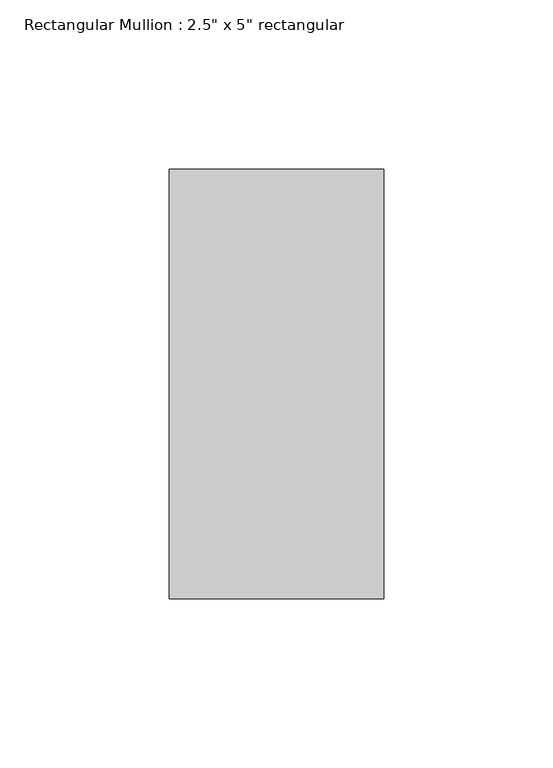
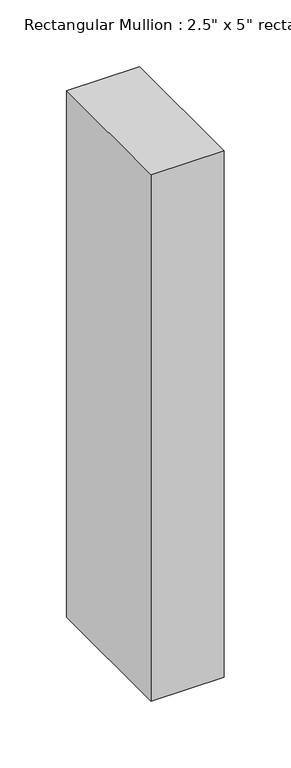
"""IFC4 building model written with IfcOpenShell, lengths in millimetres: member geometry."""

from ifc_helpers import new_model, si_unit, frame, origin, place, context, project, spatial, polyline, outline, extrude, source, transform, mapped, element, save


def member_86d06fe4(model_context):
    return source(origin(), model_context, "Body", "SweptSolid", [
        extrude(outline(polyline([(0.0, 63.5), (0.0, -63.5), (-63.5, -63.5), (-63.5, 63.5), (0.0, 63.5)])), frame((0.0, 0.0, -482.6), z_axis=(0.0, 0.0, 1.0), x_axis=(1.0, 0.0, 0.0)), (0.0, 0.0, 1.0), 482.6),
    ])


if __name__ == "__main__":
    model = new_model("IFC4")
    model_context = context("Model", 3, world=origin())
    ifc_project = project(units=[si_unit("LENGTHUNIT", "METRE", prefix="MILLI")], contexts=[model_context])
    site = spatial("IfcSite", under=ifc_project)
    building = spatial("IfcBuilding", under=site)
    placement = place(None, origin())
    member_shape = member_86d06fe4(model_context)
    element("IfcMember", 1, ObjectType="Rectangular Mullion : 2.5\" x 5\" rectangular", at=placement, inside=building, context=model_context, shape_type="MappedRepresentation", body=[
        mapped(member_shape, transform((0.0, 0.0, 0.0), x_axis=(1.0, 0.0, 0.0), y_axis=(0.0, 1.0, 0.0), z_axis=(0.0, 0.0, 1.0))),
    ])
    save(model, "model.ifc")

# Revit data of these elements
# Type "Rectangular Mullion : 2.5\" x 5\" rectangular"
#   built-in parameter 1007304 = 0.416667 (stored number, unit not read)
#   built-in parameter 1007301 = 0.104167 (stored number, unit not read)
#   built-in parameter 1007300 = 0.104167 (stored number, unit not read)
# Element 1 (IfcMember, "Rectangular Mullion : 2.5\" x 5\" rectangular")
#   Materials on its faces: "Rectangle 1 sq"
# Materials
#   "Rectangle 1 sq": class "Generic", colour RGB 120 120 120, transparency 0, Cost = 0
